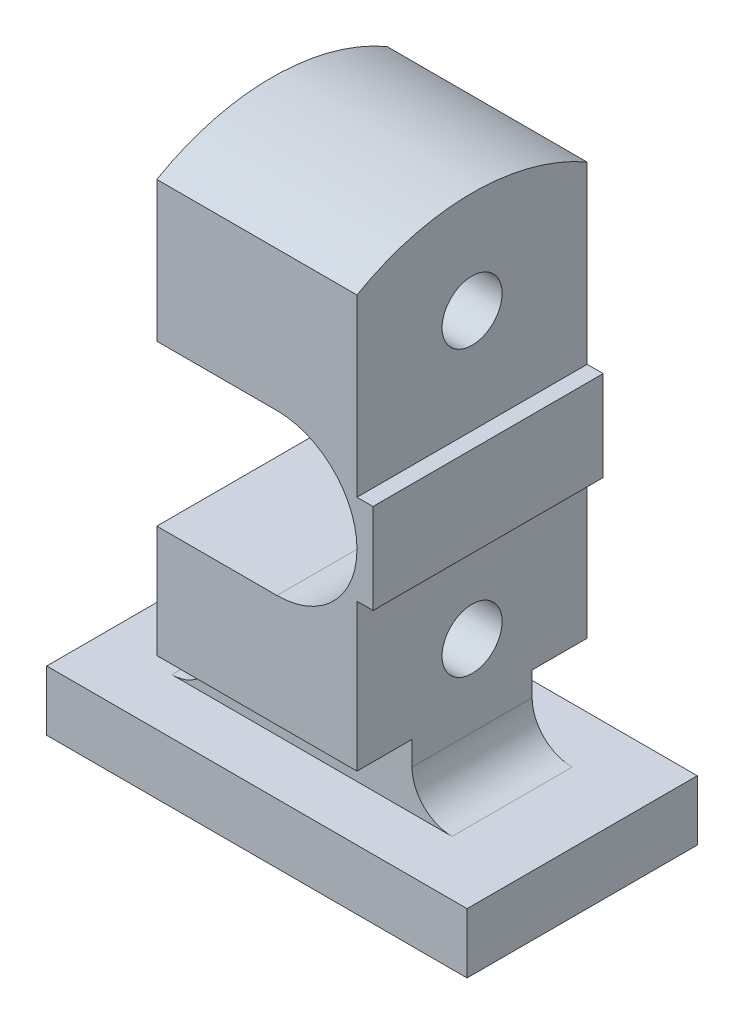
ISO-10303-21;
HEADER;
FILE_DESCRIPTION(('STEP AP214'),'2;1');
FILE_NAME('part.step','',(''),(''),'','','');
FILE_SCHEMA(('AUTOMOTIVE_DESIGN { 1 0 10303 214 1 1 1 1 }'));
ENDSEC;
DATA;
#1=APPLICATION_CONTEXT('core data for automotive mechanical design processes');
#2=APPLICATION_PROTOCOL_DEFINITION('international standard','automotive_design',2000,#1);
#3=PRODUCT_CONTEXT('',#1,'mechanical');
#4=PRODUCT('Part','Part','',(#3));
#5=PRODUCT_RELATED_PRODUCT_CATEGORY('part','',(#4));
#6=PRODUCT_DEFINITION_FORMATION('','',#4);
#7=PRODUCT_DEFINITION_CONTEXT('part definition',#1,'design');
#8=PRODUCT_DEFINITION('design','',#6,#7);
#9=PRODUCT_DEFINITION_SHAPE('','',#8);
#10=(LENGTH_UNIT() NAMED_UNIT(*) SI_UNIT(.MILLI.,.METRE.));
#11=(NAMED_UNIT(*) PLANE_ANGLE_UNIT() SI_UNIT($,.RADIAN.));
#12=(NAMED_UNIT(*) SI_UNIT($,.STERADIAN.) SOLID_ANGLE_UNIT());
#13=UNCERTAINTY_MEASURE_WITH_UNIT(LENGTH_MEASURE(1.E-05),#10,'distance_accuracy_value','');
#14=(GEOMETRIC_REPRESENTATION_CONTEXT(3) GLOBAL_UNCERTAINTY_ASSIGNED_CONTEXT((#13)) GLOBAL_UNIT_ASSIGNED_CONTEXT((#10,
#11,#12)) REPRESENTATION_CONTEXT('',''));
#15=CARTESIAN_POINT('',(0.,0.,0.));
#16=DIRECTION('',(0.,0.,1.));
#17=DIRECTION('',(1.,0.,0.));
#18=AXIS2_PLACEMENT_3D('',#15,#16,#17);
#19=CARTESIAN_POINT('',(0.,30.,0.));
#20=DIRECTION('',(0.,-1.,0.));
#21=DIRECTION('',(0.,0.,-1.));
#22=AXIS2_PLACEMENT_3D('',#19,#20,#21);
#23=PLANE('',#22);
#24=DIRECTION('',(0.,0.,-1.));
#25=VECTOR('',#24,1.);
#26=CARTESIAN_POINT('',(105.,30.,57.5));
#27=LINE('',#26,#25);
#28=CARTESIAN_POINT('',(105.,30.,57.5));
#29=VERTEX_POINT('',#28);
#30=CARTESIAN_POINT('',(105.,30.,-57.5));
#31=VERTEX_POINT('',#30);
#32=EDGE_CURVE('E323',#29,#31,#27,.T.);
#33=ORIENTED_EDGE('',*,*,#32,.T.);
#34=DIRECTION('',(-1.,0.,0.));
#35=VECTOR('',#34,1.);
#36=CARTESIAN_POINT('',(-105.,30.,-57.5));
#37=LINE('',#36,#35);
#38=CARTESIAN_POINT('',(-105.,30.,-57.5));
#39=VERTEX_POINT('',#38);
#40=EDGE_CURVE('E328',#31,#39,#37,.T.);
#41=ORIENTED_EDGE('',*,*,#40,.T.);
#42=DIRECTION('',(0.,0.,1.));
#43=VECTOR('',#42,1.);
#44=CARTESIAN_POINT('',(-105.,30.,57.5));
#45=LINE('',#44,#43);
#46=CARTESIAN_POINT('',(-105.,30.,57.5));
#47=VERTEX_POINT('',#46);
#48=EDGE_CURVE('E333',#39,#47,#45,.T.);
#49=ORIENTED_EDGE('',*,*,#48,.T.);
#50=DIRECTION('',(1.,0.,0.));
#51=VECTOR('',#50,1.);
#52=CARTESIAN_POINT('',(-105.,30.,57.5));
#53=LINE('',#52,#51);
#54=EDGE_CURVE('E332',#47,#29,#53,.T.);
#55=ORIENTED_EDGE('',*,*,#54,.T.);
#56=EDGE_LOOP('',(#33,#41,#49,#55));
#57=FACE_BOUND('',#56,.T.);
#58=DIRECTION('',(-1.,0.,0.));
#59=VECTOR('',#58,1.);
#60=CARTESIAN_POINT('',(-50.,30.,-30.));
#61=LINE('',#60,#59);
#62=CARTESIAN_POINT('',(70.,30.,-30.));
#63=VERTEX_POINT('',#62);
#64=CARTESIAN_POINT('',(-70.,30.,-30.));
#65=VERTEX_POINT('',#64);
#66=EDGE_CURVE('E303',#63,#65,#61,.T.);
#67=ORIENTED_EDGE('',*,*,#66,.F.);
#68=DIRECTION('',(0.,0.,-1.));
#69=VECTOR('',#68,1.);
#70=CARTESIAN_POINT('',(70.,30.,30.));
#71=LINE('',#70,#69);
#72=CARTESIAN_POINT('',(70.,30.,30.));
#73=VERTEX_POINT('',#72);
#74=EDGE_CURVE('E359',#63,#73,#71,.F.);
#75=ORIENTED_EDGE('',*,*,#74,.T.);
#76=DIRECTION('',(1.,0.,0.));
#77=VECTOR('',#76,1.);
#78=CARTESIAN_POINT('',(-50.,30.,30.));
#79=LINE('',#78,#77);
#80=CARTESIAN_POINT('',(-70.,30.,30.));
#81=VERTEX_POINT('',#80);
#82=EDGE_CURVE('E308',#81,#73,#79,.T.);
#83=ORIENTED_EDGE('',*,*,#82,.F.);
#84=DIRECTION('',(0.,0.,1.));
#85=VECTOR('',#84,1.);
#86=CARTESIAN_POINT('',(-70.,30.,-30.));
#87=LINE('',#86,#85);
#88=EDGE_CURVE('E357',#81,#65,#87,.F.);
#89=ORIENTED_EDGE('',*,*,#88,.T.);
#90=EDGE_LOOP('',(#67,#75,#83,#89));
#91=FACE_BOUND('',#90,.T.);
#92=ADVANCED_FACE('F39',(#57,#91),#23,.F.);
#93=CARTESIAN_POINT('',(105.,30.,57.5));
#94=DIRECTION('',(-1.,0.,0.));
#95=DIRECTION('',(0.,0.,1.));
#96=AXIS2_PLACEMENT_3D('',#93,#94,#95);
#97=PLANE('',#96);
#98=DIRECTION('',(0.,0.,-1.));
#99=VECTOR('',#98,1.);
#100=CARTESIAN_POINT('',(105.,0.,57.5));
#101=LINE('',#100,#99);
#102=CARTESIAN_POINT('',(105.,0.,57.5));
#103=VERTEX_POINT('',#102);
#104=CARTESIAN_POINT('',(105.,0.,-57.5));
#105=VERTEX_POINT('',#104);
#106=EDGE_CURVE('E321',#103,#105,#101,.T.);
#107=ORIENTED_EDGE('',*,*,#106,.T.);
#108=DIRECTION('',(0.,-1.,0.));
#109=VECTOR('',#108,1.);
#110=CARTESIAN_POINT('',(105.,30.,-57.5));
#111=LINE('',#110,#109);
#112=EDGE_CURVE('E353',#31,#105,#111,.T.);
#113=ORIENTED_EDGE('',*,*,#112,.F.);
#114=ORIENTED_EDGE('',*,*,#32,.F.);
#115=DIRECTION('',(0.,-1.,0.));
#116=VECTOR('',#115,1.);
#117=CARTESIAN_POINT('',(105.,30.,57.5));
#118=LINE('',#117,#116);
#119=EDGE_CURVE('E331',#29,#103,#118,.T.);
#120=ORIENTED_EDGE('',*,*,#119,.T.);
#121=EDGE_LOOP('',(#107,#113,#114,#120));
#122=FACE_BOUND('',#121,.T.);
#123=ADVANCED_FACE('F441',(#122),#97,.F.);
#124=CARTESIAN_POINT('',(-105.,30.,-57.5));
#125=DIRECTION('',(0.,0.,1.));
#126=DIRECTION('',(1.,0.,0.));
#127=AXIS2_PLACEMENT_3D('',#124,#125,#126);
#128=PLANE('',#127);
#129=DIRECTION('',(-1.,0.,0.));
#130=VECTOR('',#129,1.);
#131=CARTESIAN_POINT('',(-105.,0.,-57.5));
#132=LINE('',#131,#130);
#133=CARTESIAN_POINT('',(-105.,0.,-57.5));
#134=VERTEX_POINT('',#133);
#135=EDGE_CURVE('E336',#105,#134,#132,.T.);
#136=ORIENTED_EDGE('',*,*,#135,.T.);
#137=DIRECTION('',(0.,-1.,0.));
#138=VECTOR('',#137,1.);
#139=CARTESIAN_POINT('',(-105.,30.,-57.5));
#140=LINE('',#139,#138);
#141=EDGE_CURVE('E348',#39,#134,#140,.T.);
#142=ORIENTED_EDGE('',*,*,#141,.F.);
#143=ORIENTED_EDGE('',*,*,#40,.F.);
#144=ORIENTED_EDGE('',*,*,#112,.T.);
#145=EDGE_LOOP('',(#136,#142,#143,#144));
#146=FACE_BOUND('',#145,.T.);
#147=ADVANCED_FACE('F446',(#146),#128,.F.);
#148=CARTESIAN_POINT('',(-105.,30.,57.5));
#149=DIRECTION('',(1.,0.,0.));
#150=DIRECTION('',(0.,0.,-1.));
#151=AXIS2_PLACEMENT_3D('',#148,#149,#150);
#152=PLANE('',#151);
#153=DIRECTION('',(0.,0.,1.));
#154=VECTOR('',#153,1.);
#155=CARTESIAN_POINT('',(-105.,0.,57.5));
#156=LINE('',#155,#154);
#157=CARTESIAN_POINT('',(-105.,0.,57.5));
#158=VERTEX_POINT('',#157);
#159=EDGE_CURVE('E338',#134,#158,#156,.T.);
#160=ORIENTED_EDGE('',*,*,#159,.T.);
#161=DIRECTION('',(0.,-1.,0.));
#162=VECTOR('',#161,1.);
#163=CARTESIAN_POINT('',(-105.,30.,57.5));
#164=LINE('',#163,#162);
#165=EDGE_CURVE('E343',#47,#158,#164,.T.);
#166=ORIENTED_EDGE('',*,*,#165,.F.);
#167=ORIENTED_EDGE('',*,*,#48,.F.);
#168=ORIENTED_EDGE('',*,*,#141,.T.);
#169=EDGE_LOOP('',(#160,#166,#167,#168));
#170=FACE_BOUND('',#169,.T.);
#171=ADVANCED_FACE('F463',(#170),#152,.F.);
#172=CARTESIAN_POINT('',(-105.,30.,57.5));
#173=DIRECTION('',(0.,0.,-1.));
#174=DIRECTION('',(-1.,0.,0.));
#175=AXIS2_PLACEMENT_3D('',#172,#173,#174);
#176=PLANE('',#175);
#177=DIRECTION('',(1.,0.,0.));
#178=VECTOR('',#177,1.);
#179=CARTESIAN_POINT('',(-105.,0.,57.5));
#180=LINE('',#179,#178);
#181=EDGE_CURVE('E329',#158,#103,#180,.T.);
#182=ORIENTED_EDGE('',*,*,#181,.T.);
#183=ORIENTED_EDGE('',*,*,#119,.F.);
#184=ORIENTED_EDGE('',*,*,#54,.F.);
#185=ORIENTED_EDGE('',*,*,#165,.T.);
#186=EDGE_LOOP('',(#182,#183,#184,#185));
#187=FACE_BOUND('',#186,.T.);
#188=ADVANCED_FACE('F460',(#187),#176,.F.);
#189=CARTESIAN_POINT('',(0.,0.,0.));
#190=DIRECTION('',(0.,-1.,0.));
#191=DIRECTION('',(0.,0.,-1.));
#192=AXIS2_PLACEMENT_3D('',#189,#190,#191);
#193=PLANE('',#192);
#194=ORIENTED_EDGE('',*,*,#106,.F.);
#195=ORIENTED_EDGE('',*,*,#181,.F.);
#196=ORIENTED_EDGE('',*,*,#159,.F.);
#197=ORIENTED_EDGE('',*,*,#135,.F.);
#198=EDGE_LOOP('',(#194,#195,#196,#197));
#199=FACE_BOUND('',#198,.T.);
#200=ADVANCED_FACE('F453',(#199),#193,.T.);
#201=CARTESIAN_POINT('',(50.,62.,30.));
#202=DIRECTION('',(-1.,0.,0.));
#203=DIRECTION('',(0.,0.,1.));
#204=AXIS2_PLACEMENT_3D('',#201,#202,#203);
#205=PLANE('',#204);
#206=CARTESIAN_POINT('',(50.,90.5,0.));
#207=DIRECTION('',(-1.,0.,0.));
#208=DIRECTION('',(0.,0.,1.));
#209=AXIS2_PLACEMENT_3D('',#206,#207,#208);
#210=CIRCLE('',#209,15.);
#211=CARTESIAN_POINT('',(50.,90.5,15.));
#212=VERTEX_POINT('',#211);
#213=EDGE_CURVE('E225',#212,#212,#210,.T.);
#214=ORIENTED_EDGE('',*,*,#213,.T.);
#215=EDGE_LOOP('',(#214));
#216=FACE_BOUND('',#215,.T.);
#217=DIRECTION('',(0.,-1.,0.));
#218=VECTOR('',#217,1.);
#219=CARTESIAN_POINT('',(50.,62.,30.));
#220=LINE('',#219,#218);
#221=CARTESIAN_POINT('',(50.,62.,30.));
#222=VERTEX_POINT('',#221);
#223=CARTESIAN_POINT('',(50.,50.,30.));
#224=VERTEX_POINT('',#223);
#225=EDGE_CURVE('E311',#222,#224,#220,.T.);
#226=ORIENTED_EDGE('',*,*,#225,.T.);
#227=DIRECTION('',(0.,0.,-1.));
#228=VECTOR('',#227,1.);
#229=CARTESIAN_POINT('',(50.,50.,-30.));
#230=LINE('',#229,#228);
#231=CARTESIAN_POINT('',(50.,50.,-30.));
#232=VERTEX_POINT('',#231);
#233=EDGE_CURVE('E355',#224,#232,#230,.T.);
#234=ORIENTED_EDGE('',*,*,#233,.T.);
#235=DIRECTION('',(0.,-1.,0.));
#236=VECTOR('',#235,1.);
#237=CARTESIAN_POINT('',(50.,62.,-30.));
#238=LINE('',#237,#236);
#239=CARTESIAN_POINT('',(50.,62.,-30.));
#240=VERTEX_POINT('',#239);
#241=EDGE_CURVE('E322',#240,#232,#238,.T.);
#242=ORIENTED_EDGE('',*,*,#241,.F.);
#243=DIRECTION('',(0.,0.,-1.));
#244=VECTOR('',#243,1.);
#245=CARTESIAN_POINT('',(50.,62.,57.5));
#246=LINE('',#245,#244);
#247=CARTESIAN_POINT('',(50.,62.,-57.5));
#248=VERTEX_POINT('',#247);
#249=EDGE_CURVE('E299',#240,#248,#246,.T.);
#250=ORIENTED_EDGE('',*,*,#249,.T.);
#251=DIRECTION('',(0.,1.,0.));
#252=VECTOR('',#251,1.);
#253=CARTESIAN_POINT('',(50.,118.,-57.5));
#254=LINE('',#253,#252);
#255=CARTESIAN_POINT('',(50.,135.5,-57.5));
#256=VERTEX_POINT('',#255);
#257=EDGE_CURVE('E257',#248,#256,#254,.T.);
#258=ORIENTED_EDGE('',*,*,#257,.T.);
#259=DIRECTION('',(0.,0.,-1.));
#260=VECTOR('',#259,1.);
#261=CARTESIAN_POINT('',(50.,135.5,57.5));
#262=LINE('',#261,#260);
#263=CARTESIAN_POINT('',(50.,135.5,57.5));
#264=VERTEX_POINT('',#263);
#265=EDGE_CURVE('E298',#264,#256,#262,.T.);
#266=ORIENTED_EDGE('',*,*,#265,.F.);
#267=DIRECTION('',(0.,1.,0.));
#268=VECTOR('',#267,1.);
#269=CARTESIAN_POINT('',(50.,62.,57.5));
#270=LINE('',#269,#268);
#271=CARTESIAN_POINT('',(50.,62.,57.5));
#272=VERTEX_POINT('',#271);
#273=EDGE_CURVE('E233',#272,#264,#270,.T.);
#274=ORIENTED_EDGE('',*,*,#273,.F.);
#275=EDGE_CURVE('E297',#272,#222,#246,.T.);
#276=ORIENTED_EDGE('',*,*,#275,.T.);
#277=EDGE_LOOP('',(#226,#234,#242,#250,#258,#266,#274,#276));
#278=FACE_BOUND('',#277,.T.);
#279=ADVANCED_FACE('F378',(#216,#278),#205,.F.);
#280=CARTESIAN_POINT('',(-50.,62.,-30.));
#281=DIRECTION('',(0.,0.,1.));
#282=DIRECTION('',(1.,0.,0.));
#283=AXIS2_PLACEMENT_3D('',#280,#281,#282);
#284=PLANE('',#283);
#285=ORIENTED_EDGE('',*,*,#66,.T.);
#286=CARTESIAN_POINT('',(-70.,50.,-30.));
#287=DIRECTION('',(0.,0.,1.));
#288=DIRECTION('',(1.,0.,0.));
#289=AXIS2_PLACEMENT_3D('',#286,#287,#288);
#290=CIRCLE('',#289,20.);
#291=CARTESIAN_POINT('',(-50.,50.,-30.));
#292=VERTEX_POINT('',#291);
#293=EDGE_CURVE('E11',#65,#292,#290,.T.);
#294=ORIENTED_EDGE('',*,*,#293,.T.);
#295=DIRECTION('',(0.,-1.,0.));
#296=VECTOR('',#295,1.);
#297=CARTESIAN_POINT('',(-50.,62.,-30.));
#298=LINE('',#297,#296);
#299=CARTESIAN_POINT('',(-50.,62.,-30.));
#300=VERTEX_POINT('',#299);
#301=EDGE_CURVE('E316',#300,#292,#298,.T.);
#302=ORIENTED_EDGE('',*,*,#301,.F.);
#303=DIRECTION('',(-1.,0.,0.));
#304=VECTOR('',#303,1.);
#305=CARTESIAN_POINT('',(-50.,62.,-30.));
#306=LINE('',#305,#304);
#307=EDGE_CURVE('E302',#240,#300,#306,.T.);
#308=ORIENTED_EDGE('',*,*,#307,.F.);
#309=ORIENTED_EDGE('',*,*,#241,.T.);
#310=CARTESIAN_POINT('',(70.,50.,-30.));
#311=DIRECTION('',(0.,0.,1.));
#312=DIRECTION('',(1.,0.,0.));
#313=AXIS2_PLACEMENT_3D('',#310,#311,#312);
#314=CIRCLE('',#313,20.);
#315=EDGE_CURVE('E362',#232,#63,#314,.T.);
#316=ORIENTED_EDGE('',*,*,#315,.T.);
#317=EDGE_LOOP('',(#285,#294,#302,#308,#309,#316));
#318=FACE_BOUND('',#317,.T.);
#319=ADVANCED_FACE('F392',(#318),#284,.F.);
#320=CARTESIAN_POINT('',(-50.,62.,30.));
#321=DIRECTION('',(1.,0.,0.));
#322=DIRECTION('',(0.,0.,-1.));
#323=AXIS2_PLACEMENT_3D('',#320,#321,#322);
#324=PLANE('',#323);
#325=CARTESIAN_POINT('',(-50.,90.5,0.));
#326=DIRECTION('',(-1.,0.,0.));
#327=DIRECTION('',(0.,0.,1.));
#328=AXIS2_PLACEMENT_3D('',#325,#326,#327);
#329=CIRCLE('',#328,15.);
#330=CARTESIAN_POINT('',(-50.,90.5,15.));
#331=VERTEX_POINT('',#330);
#332=EDGE_CURVE('E217',#331,#331,#329,.T.);
#333=ORIENTED_EDGE('',*,*,#332,.F.);
#334=EDGE_LOOP('',(#333));
#335=FACE_BOUND('',#334,.T.);
#336=ORIENTED_EDGE('',*,*,#301,.T.);
#337=DIRECTION('',(0.,0.,1.));
#338=VECTOR('',#337,1.);
#339=CARTESIAN_POINT('',(-50.,50.,30.));
#340=LINE('',#339,#338);
#341=CARTESIAN_POINT('',(-50.,50.,30.));
#342=VERTEX_POINT('',#341);
#343=EDGE_CURVE('E361',#292,#342,#340,.T.);
#344=ORIENTED_EDGE('',*,*,#343,.T.);
#345=DIRECTION('',(0.,-1.,0.));
#346=VECTOR('',#345,1.);
#347=CARTESIAN_POINT('',(-50.,62.,30.));
#348=LINE('',#347,#346);
#349=CARTESIAN_POINT('',(-50.,62.,30.));
#350=VERTEX_POINT('',#349);
#351=EDGE_CURVE('E317',#350,#342,#348,.T.);
#352=ORIENTED_EDGE('',*,*,#351,.F.);
#353=DIRECTION('',(0.,0.,-1.));
#354=VECTOR('',#353,1.);
#355=CARTESIAN_POINT('',(-50.,62.,57.5));
#356=LINE('',#355,#354);
#357=CARTESIAN_POINT('',(-50.,62.,57.5));
#358=VERTEX_POINT('',#357);
#359=EDGE_CURVE('E271',#358,#350,#356,.T.);
#360=ORIENTED_EDGE('',*,*,#359,.F.);
#361=DIRECTION('',(0.,-1.,0.));
#362=VECTOR('',#361,1.);
#363=CARTESIAN_POINT('',(-50.,118.,57.5));
#364=LINE('',#363,#362);
#365=CARTESIAN_POINT('',(-50.,118.,57.5));
#366=VERTEX_POINT('',#365);
#367=EDGE_CURVE('E252',#366,#358,#364,.T.);
#368=ORIENTED_EDGE('',*,*,#367,.F.);
#369=DIRECTION('',(0.,0.,-1.));
#370=VECTOR('',#369,1.);
#371=CARTESIAN_POINT('',(-50.,118.,57.5));
#372=LINE('',#371,#370);
#373=CARTESIAN_POINT('',(-50.,118.,-57.5));
#374=VERTEX_POINT('',#373);
#375=EDGE_CURVE('E277',#366,#374,#372,.T.);
#376=ORIENTED_EDGE('',*,*,#375,.T.);
#377=DIRECTION('',(0.,-1.,0.));
#378=VECTOR('',#377,1.);
#379=CARTESIAN_POINT('',(-50.,118.,-57.5));
#380=LINE('',#379,#378);
#381=CARTESIAN_POINT('',(-50.,62.,-57.5));
#382=VERTEX_POINT('',#381);
#383=EDGE_CURVE('E235',#374,#382,#380,.T.);
#384=ORIENTED_EDGE('',*,*,#383,.T.);
#385=EDGE_CURVE('E254',#300,#382,#356,.T.);
#386=ORIENTED_EDGE('',*,*,#385,.F.);
#387=EDGE_LOOP('',(#336,#344,#352,#360,#368,#376,#384,#386));
#388=FACE_BOUND('',#387,.T.);
#389=ADVANCED_FACE('F386',(#335,#388),#324,.F.);
#390=CARTESIAN_POINT('',(-50.,62.,30.));
#391=DIRECTION('',(0.,0.,-1.));
#392=DIRECTION('',(-1.,0.,0.));
#393=AXIS2_PLACEMENT_3D('',#390,#391,#392);
#394=PLANE('',#393);
#395=ORIENTED_EDGE('',*,*,#82,.T.);
#396=CARTESIAN_POINT('',(70.,50.,30.));
#397=DIRECTION('',(0.,0.,-1.));
#398=DIRECTION('',(-1.,0.,0.));
#399=AXIS2_PLACEMENT_3D('',#396,#397,#398);
#400=CIRCLE('',#399,20.);
#401=EDGE_CURVE('E368',#73,#224,#400,.T.);
#402=ORIENTED_EDGE('',*,*,#401,.T.);
#403=ORIENTED_EDGE('',*,*,#225,.F.);
#404=DIRECTION('',(1.,0.,0.));
#405=VECTOR('',#404,1.);
#406=CARTESIAN_POINT('',(-50.,62.,30.));
#407=LINE('',#406,#405);
#408=EDGE_CURVE('E310',#350,#222,#407,.T.);
#409=ORIENTED_EDGE('',*,*,#408,.F.);
#410=ORIENTED_EDGE('',*,*,#351,.T.);
#411=CARTESIAN_POINT('',(-70.,50.,30.));
#412=DIRECTION('',(0.,0.,-1.));
#413=DIRECTION('',(-1.,0.,0.));
#414=AXIS2_PLACEMENT_3D('',#411,#412,#413);
#415=CIRCLE('',#414,20.);
#416=EDGE_CURVE('E50',#342,#81,#415,.T.);
#417=ORIENTED_EDGE('',*,*,#416,.T.);
#418=EDGE_LOOP('',(#395,#402,#403,#409,#410,#417));
#419=FACE_BOUND('',#418,.T.);
#420=ADVANCED_FACE('F369',(#419),#394,.F.);
#421=CARTESIAN_POINT('',(70.,50.,30.));
#422=DIRECTION('',(0.,0.,1.));
#423=DIRECTION('',(1.,0.,0.));
#424=AXIS2_PLACEMENT_3D('',#421,#422,#423);
#425=CYLINDRICAL_SURFACE('',#424,20.);
#426=ORIENTED_EDGE('',*,*,#401,.F.);
#427=ORIENTED_EDGE('',*,*,#74,.F.);
#428=ORIENTED_EDGE('',*,*,#315,.F.);
#429=ORIENTED_EDGE('',*,*,#233,.F.);
#430=EDGE_LOOP('',(#426,#427,#428,#429));
#431=FACE_BOUND('',#430,.T.);
#432=ADVANCED_FACE('F380',(#431),#425,.F.);
#433=CARTESIAN_POINT('',(-70.,50.,30.));
#434=DIRECTION('',(0.,0.,-1.));
#435=DIRECTION('',(-1.,0.,0.));
#436=AXIS2_PLACEMENT_3D('',#433,#434,#435);
#437=CYLINDRICAL_SURFACE('',#436,20.);
#438=ORIENTED_EDGE('',*,*,#293,.F.);
#439=ORIENTED_EDGE('',*,*,#88,.F.);
#440=ORIENTED_EDGE('',*,*,#416,.F.);
#441=ORIENTED_EDGE('',*,*,#343,.F.);
#442=EDGE_LOOP('',(#438,#439,#440,#441));
#443=FACE_BOUND('',#442,.T.);
#444=ADVANCED_FACE('F41',(#443),#437,.F.);
#445=CARTESIAN_POINT('',(-50.,62.,57.5));
#446=DIRECTION('',(0.,1.,0.));
#447=DIRECTION('',(0.,0.,1.));
#448=AXIS2_PLACEMENT_3D('',#445,#446,#447);
#449=PLANE('',#448);
#450=ORIENTED_EDGE('',*,*,#249,.F.);
#451=ORIENTED_EDGE('',*,*,#307,.T.);
#452=ORIENTED_EDGE('',*,*,#385,.T.);
#453=DIRECTION('',(1.,0.,0.));
#454=VECTOR('',#453,1.);
#455=CARTESIAN_POINT('',(-50.,62.,-57.5));
#456=LINE('',#455,#454);
#457=EDGE_CURVE('E227',#382,#248,#456,.T.);
#458=ORIENTED_EDGE('',*,*,#457,.T.);
#459=EDGE_LOOP('',(#450,#451,#452,#458));
#460=FACE_BOUND('',#459,.T.);
#461=ADVANCED_FACE('F394',(#460),#449,.F.);
#462=ORIENTED_EDGE('',*,*,#359,.T.);
#463=ORIENTED_EDGE('',*,*,#408,.T.);
#464=ORIENTED_EDGE('',*,*,#275,.F.);
#465=DIRECTION('',(1.,0.,0.));
#466=VECTOR('',#465,1.);
#467=CARTESIAN_POINT('',(-50.,62.,57.5));
#468=LINE('',#467,#466);
#469=EDGE_CURVE('E226',#358,#272,#468,.T.);
#470=ORIENTED_EDGE('',*,*,#469,.F.);
#471=EDGE_LOOP('',(#462,#463,#464,#470));
#472=FACE_BOUND('',#471,.T.);
#473=ADVANCED_FACE('F383',(#472),#449,.F.);
#474=CARTESIAN_POINT('',(50.,135.5,57.5));
#475=DIRECTION('',(0.,1.,0.));
#476=DIRECTION('',(0.,0.,1.));
#477=AXIS2_PLACEMENT_3D('',#474,#475,#476);
#478=PLANE('',#477);
#479=DIRECTION('',(1.,0.,0.));
#480=VECTOR('',#479,1.);
#481=CARTESIAN_POINT('',(50.,135.5,-57.5));
#482=LINE('',#481,#480);
#483=CARTESIAN_POINT('',(58.,135.5,-57.5));
#484=VERTEX_POINT('',#483);
#485=EDGE_CURVE('E259',#256,#484,#482,.T.);
#486=ORIENTED_EDGE('',*,*,#485,.T.);
#487=DIRECTION('',(0.,0.,-1.));
#488=VECTOR('',#487,1.);
#489=CARTESIAN_POINT('',(58.,135.5,57.5));
#490=LINE('',#489,#488);
#491=CARTESIAN_POINT('',(58.,135.5,57.5));
#492=VERTEX_POINT('',#491);
#493=EDGE_CURVE('E291',#492,#484,#490,.T.);
#494=ORIENTED_EDGE('',*,*,#493,.F.);
#495=DIRECTION('',(1.,0.,0.));
#496=VECTOR('',#495,1.);
#497=CARTESIAN_POINT('',(50.,135.5,57.5));
#498=LINE('',#497,#496);
#499=EDGE_CURVE('E234',#264,#492,#498,.T.);
#500=ORIENTED_EDGE('',*,*,#499,.F.);
#501=ORIENTED_EDGE('',*,*,#265,.T.);
#502=EDGE_LOOP('',(#486,#494,#500,#501));
#503=FACE_BOUND('',#502,.T.);
#504=ADVANCED_FACE('F405',(#503),#478,.F.);
#505=CARTESIAN_POINT('',(58.,135.5,57.5));
#506=DIRECTION('',(-1.,0.,0.));
#507=DIRECTION('',(0.,0.,1.));
#508=AXIS2_PLACEMENT_3D('',#505,#506,#507);
#509=PLANE('',#508);
#510=DIRECTION('',(0.,1.,0.));
#511=VECTOR('',#510,1.);
#512=CARTESIAN_POINT('',(58.,135.5,-57.5));
#513=LINE('',#512,#511);
#514=CARTESIAN_POINT('',(58.,180.5,-57.5));
#515=VERTEX_POINT('',#514);
#516=EDGE_CURVE('E258',#484,#515,#513,.T.);
#517=ORIENTED_EDGE('',*,*,#516,.T.);
#518=DIRECTION('',(0.,0.,-1.));
#519=VECTOR('',#518,1.);
#520=CARTESIAN_POINT('',(58.,180.5,57.5));
#521=LINE('',#520,#519);
#522=CARTESIAN_POINT('',(58.,180.5,57.5));
#523=VERTEX_POINT('',#522);
#524=EDGE_CURVE('E286',#523,#515,#521,.T.);
#525=ORIENTED_EDGE('',*,*,#524,.F.);
#526=DIRECTION('',(0.,1.,0.));
#527=VECTOR('',#526,1.);
#528=CARTESIAN_POINT('',(58.,135.5,57.5));
#529=LINE('',#528,#527);
#530=EDGE_CURVE('E236',#492,#523,#529,.T.);
#531=ORIENTED_EDGE('',*,*,#530,.F.);
#532=ORIENTED_EDGE('',*,*,#493,.T.);
#533=EDGE_LOOP('',(#517,#525,#531,#532));
#534=FACE_BOUND('',#533,.T.);
#535=ADVANCED_FACE('F407',(#534),#509,.F.);
#536=CARTESIAN_POINT('',(58.,180.5,57.5));
#537=DIRECTION('',(0.,-1.,0.));
#538=DIRECTION('',(0.,0.,-1.));
#539=AXIS2_PLACEMENT_3D('',#536,#537,#538);
#540=PLANE('',#539);
#541=DIRECTION('',(-1.,0.,0.));
#542=VECTOR('',#541,1.);
#543=CARTESIAN_POINT('',(58.,180.5,-57.5));
#544=LINE('',#543,#542);
#545=CARTESIAN_POINT('',(50.,180.5,-57.5));
#546=VERTEX_POINT('',#545);
#547=EDGE_CURVE('E265',#515,#546,#544,.T.);
#548=ORIENTED_EDGE('',*,*,#547,.T.);
#549=DIRECTION('',(0.,0.,-1.));
#550=VECTOR('',#549,1.);
#551=CARTESIAN_POINT('',(50.,180.5,57.5));
#552=LINE('',#551,#550);
#553=CARTESIAN_POINT('',(50.,180.5,57.5));
#554=VERTEX_POINT('',#553);
#555=EDGE_CURVE('E289',#554,#546,#552,.T.);
#556=ORIENTED_EDGE('',*,*,#555,.F.);
#557=DIRECTION('',(-1.,0.,0.));
#558=VECTOR('',#557,1.);
#559=CARTESIAN_POINT('',(58.,180.5,57.5));
#560=LINE('',#559,#558);
#561=EDGE_CURVE('E238',#523,#554,#560,.T.);
#562=ORIENTED_EDGE('',*,*,#561,.F.);
#563=ORIENTED_EDGE('',*,*,#524,.T.);
#564=EDGE_LOOP('',(#548,#556,#562,#563));
#565=FACE_BOUND('',#564,.T.);
#566=ADVANCED_FACE('F429',(#565),#540,.F.);
#567=CARTESIAN_POINT('',(50.,198.,57.5));
#568=DIRECTION('',(-1.,0.,0.));
#569=DIRECTION('',(0.,0.,1.));
#570=AXIS2_PLACEMENT_3D('',#567,#568,#569);
#571=PLANE('',#570);
#572=CARTESIAN_POINT('',(50.,232.5,0.));
#573=DIRECTION('',(-1.,0.,0.));
#574=DIRECTION('',(0.,0.,1.));
#575=AXIS2_PLACEMENT_3D('',#572,#573,#574);
#576=CIRCLE('',#575,15.);
#577=CARTESIAN_POINT('',(50.,232.5,15.));
#578=VERTEX_POINT('',#577);
#579=EDGE_CURVE('E219',#578,#578,#576,.T.);
#580=ORIENTED_EDGE('',*,*,#579,.T.);
#581=EDGE_LOOP('',(#580));
#582=FACE_BOUND('',#581,.T.);
#583=DIRECTION('',(0.,1.,0.));
#584=VECTOR('',#583,1.);
#585=CARTESIAN_POINT('',(50.,198.,-57.5));
#586=LINE('',#585,#584);
#587=CARTESIAN_POINT('',(50.,268.,-57.5));
#588=VERTEX_POINT('',#587);
#589=EDGE_CURVE('E210',#546,#588,#586,.T.);
#590=ORIENTED_EDGE('',*,*,#589,.T.);
#591=CARTESIAN_POINT('',(50.,168.40707856479,0.));
#592=DIRECTION('',(-1.,0.,0.));
#593=DIRECTION('',(0.,0.,-1.));
#594=AXIS2_PLACEMENT_3D('',#591,#592,#593);
#595=CIRCLE('',#594,115.);
#596=CARTESIAN_POINT('',(50.,268.,57.5));
#597=VERTEX_POINT('',#596);
#598=EDGE_CURVE('E207',#597,#588,#595,.T.);
#599=ORIENTED_EDGE('',*,*,#598,.F.);
#600=DIRECTION('',(0.,1.,0.));
#601=VECTOR('',#600,1.);
#602=CARTESIAN_POINT('',(50.,180.5,57.5));
#603=LINE('',#602,#601);
#604=EDGE_CURVE('E239',#554,#597,#603,.T.);
#605=ORIENTED_EDGE('',*,*,#604,.F.);
#606=ORIENTED_EDGE('',*,*,#555,.T.);
#607=EDGE_LOOP('',(#590,#599,#605,#606));
#608=FACE_BOUND('',#607,.T.);
#609=ADVANCED_FACE('F430',(#582,#608),#571,.F.);
#610=CARTESIAN_POINT('',(-50.,268.,57.5));
#611=DIRECTION('',(1.,0.,0.));
#612=DIRECTION('',(0.,0.,-1.));
#613=AXIS2_PLACEMENT_3D('',#610,#611,#612);
#614=PLANE('',#613);
#615=CARTESIAN_POINT('',(-50.,232.5,0.));
#616=DIRECTION('',(-1.,0.,0.));
#617=DIRECTION('',(0.,0.,1.));
#618=AXIS2_PLACEMENT_3D('',#615,#616,#617);
#619=CIRCLE('',#618,15.);
#620=CARTESIAN_POINT('',(-50.,232.5,15.));
#621=VERTEX_POINT('',#620);
#622=EDGE_CURVE('E214',#621,#621,#619,.T.);
#623=ORIENTED_EDGE('',*,*,#622,.F.);
#624=EDGE_LOOP('',(#623));
#625=FACE_BOUND('',#624,.T.);
#626=DIRECTION('',(0.,-1.,0.));
#627=VECTOR('',#626,1.);
#628=CARTESIAN_POINT('',(-50.,268.,-57.5));
#629=LINE('',#628,#627);
#630=CARTESIAN_POINT('',(-50.,268.,-57.5));
#631=VERTEX_POINT('',#630);
#632=CARTESIAN_POINT('',(-50.,198.,-57.5));
#633=VERTEX_POINT('',#632);
#634=EDGE_CURVE('E190',#631,#633,#629,.T.);
#635=ORIENTED_EDGE('',*,*,#634,.T.);
#636=DIRECTION('',(0.,0.,-1.));
#637=VECTOR('',#636,1.);
#638=CARTESIAN_POINT('',(-50.,198.,57.5));
#639=LINE('',#638,#637);
#640=CARTESIAN_POINT('',(-50.,198.,57.5));
#641=VERTEX_POINT('',#640);
#642=EDGE_CURVE('E281',#641,#633,#639,.T.);
#643=ORIENTED_EDGE('',*,*,#642,.F.);
#644=DIRECTION('',(0.,-1.,0.));
#645=VECTOR('',#644,1.);
#646=CARTESIAN_POINT('',(-50.,268.,57.5));
#647=LINE('',#646,#645);
#648=CARTESIAN_POINT('',(-50.,268.,57.5));
#649=VERTEX_POINT('',#648);
#650=EDGE_CURVE('E212',#649,#641,#647,.T.);
#651=ORIENTED_EDGE('',*,*,#650,.F.);
#652=CARTESIAN_POINT('',(-50.,168.40707856479,0.));
#653=DIRECTION('',(-1.,0.,0.));
#654=DIRECTION('',(0.,0.,-1.));
#655=AXIS2_PLACEMENT_3D('',#652,#653,#654);
#656=CIRCLE('',#655,115.);
#657=EDGE_CURVE('E205',#649,#631,#656,.T.);
#658=ORIENTED_EDGE('',*,*,#657,.T.);
#659=EDGE_LOOP('',(#635,#643,#651,#658));
#660=FACE_BOUND('',#659,.T.);
#661=ADVANCED_FACE('F208',(#625,#660),#614,.F.);
#662=CARTESIAN_POINT('',(-50.,198.,57.5));
#663=DIRECTION('',(0.,1.,0.));
#664=DIRECTION('',(0.,0.,1.));
#665=AXIS2_PLACEMENT_3D('',#662,#663,#664);
#666=PLANE('',#665);
#667=DIRECTION('',(1.,0.,0.));
#668=VECTOR('',#667,1.);
#669=CARTESIAN_POINT('',(-50.,198.,-57.5));
#670=LINE('',#669,#668);
#671=CARTESIAN_POINT('',(10.,198.,-57.5));
#672=VERTEX_POINT('',#671);
#673=EDGE_CURVE('E191',#633,#672,#670,.T.);
#674=ORIENTED_EDGE('',*,*,#673,.T.);
#675=DIRECTION('',(0.,0.,-1.));
#676=VECTOR('',#675,1.);
#677=CARTESIAN_POINT('',(10.,198.,57.5));
#678=LINE('',#677,#676);
#679=CARTESIAN_POINT('',(10.,198.,57.5));
#680=VERTEX_POINT('',#679);
#681=EDGE_CURVE('E285',#680,#672,#678,.T.);
#682=ORIENTED_EDGE('',*,*,#681,.F.);
#683=DIRECTION('',(1.,0.,0.));
#684=VECTOR('',#683,1.);
#685=CARTESIAN_POINT('',(-50.,198.,57.5));
#686=LINE('',#685,#684);
#687=EDGE_CURVE('E244',#641,#680,#686,.T.);
#688=ORIENTED_EDGE('',*,*,#687,.F.);
#689=ORIENTED_EDGE('',*,*,#642,.T.);
#690=EDGE_LOOP('',(#674,#682,#688,#689));
#691=FACE_BOUND('',#690,.T.);
#692=ADVANCED_FACE('F425',(#691),#666,.F.);
#693=CARTESIAN_POINT('',(10.,158.,57.5));
#694=DIRECTION('',(0.,0.,-1.));
#695=DIRECTION('',(-1.,0.,0.));
#696=AXIS2_PLACEMENT_3D('',#693,#694,#695);
#697=CYLINDRICAL_SURFACE('',#696,40.);
#698=CARTESIAN_POINT('',(10.,158.,-57.5));
#699=DIRECTION('',(0.,0.,-1.));
#700=DIRECTION('',(1.,0.,0.));
#701=AXIS2_PLACEMENT_3D('',#698,#699,#700);
#702=CIRCLE('',#701,40.);
#703=CARTESIAN_POINT('',(10.,118.,-57.5));
#704=VERTEX_POINT('',#703);
#705=EDGE_CURVE('E269',#672,#704,#702,.T.);
#706=ORIENTED_EDGE('',*,*,#705,.T.);
#707=DIRECTION('',(0.,0.,-1.));
#708=VECTOR('',#707,1.);
#709=CARTESIAN_POINT('',(10.,118.,57.5));
#710=LINE('',#709,#708);
#711=CARTESIAN_POINT('',(10.,118.,57.5));
#712=VERTEX_POINT('',#711);
#713=EDGE_CURVE('E276',#712,#704,#710,.T.);
#714=ORIENTED_EDGE('',*,*,#713,.F.);
#715=CARTESIAN_POINT('',(10.,158.,57.5));
#716=DIRECTION('',(0.,0.,-1.));
#717=DIRECTION('',(1.,0.,0.));
#718=AXIS2_PLACEMENT_3D('',#715,#716,#717);
#719=CIRCLE('',#718,40.);
#720=EDGE_CURVE('E250',#680,#712,#719,.T.);
#721=ORIENTED_EDGE('',*,*,#720,.F.);
#722=ORIENTED_EDGE('',*,*,#681,.T.);
#723=EDGE_LOOP('',(#706,#714,#721,#722));
#724=FACE_BOUND('',#723,.T.);
#725=ADVANCED_FACE('F416',(#724),#697,.F.);
#726=CARTESIAN_POINT('',(10.,118.,57.5));
#727=DIRECTION('',(0.,-1.,0.));
#728=DIRECTION('',(0.,0.,-1.));
#729=AXIS2_PLACEMENT_3D('',#726,#727,#728);
#730=PLANE('',#729);
#731=DIRECTION('',(-1.,0.,0.));
#732=VECTOR('',#731,1.);
#733=CARTESIAN_POINT('',(10.,118.,-57.5));
#734=LINE('',#733,#732);
#735=EDGE_CURVE('E270',#704,#374,#734,.T.);
#736=ORIENTED_EDGE('',*,*,#735,.T.);
#737=ORIENTED_EDGE('',*,*,#375,.F.);
#738=DIRECTION('',(-1.,0.,0.));
#739=VECTOR('',#738,1.);
#740=CARTESIAN_POINT('',(10.,118.,57.5));
#741=LINE('',#740,#739);
#742=EDGE_CURVE('E248',#712,#366,#741,.T.);
#743=ORIENTED_EDGE('',*,*,#742,.F.);
#744=ORIENTED_EDGE('',*,*,#713,.T.);
#745=EDGE_LOOP('',(#736,#737,#743,#744));
#746=FACE_BOUND('',#745,.T.);
#747=ADVANCED_FACE('F419',(#746),#730,.F.);
#748=CARTESIAN_POINT('',(10.,158.,57.5));
#749=DIRECTION('',(0.,0.,1.));
#750=DIRECTION('',(1.,0.,0.));
#751=AXIS2_PLACEMENT_3D('',#748,#749,#750);
#752=PLANE('',#751);
#753=ORIENTED_EDGE('',*,*,#469,.T.);
#754=ORIENTED_EDGE('',*,*,#273,.T.);
#755=ORIENTED_EDGE('',*,*,#499,.T.);
#756=ORIENTED_EDGE('',*,*,#530,.T.);
#757=ORIENTED_EDGE('',*,*,#561,.T.);
#758=ORIENTED_EDGE('',*,*,#604,.T.);
#759=DIRECTION('',(-1.,0.,0.));
#760=VECTOR('',#759,1.);
#761=CARTESIAN_POINT('',(50.,268.,57.5));
#762=LINE('',#761,#760);
#763=EDGE_CURVE('E245',#597,#649,#762,.T.);
#764=ORIENTED_EDGE('',*,*,#763,.T.);
#765=ORIENTED_EDGE('',*,*,#650,.T.);
#766=ORIENTED_EDGE('',*,*,#687,.T.);
#767=ORIENTED_EDGE('',*,*,#720,.T.);
#768=ORIENTED_EDGE('',*,*,#742,.T.);
#769=ORIENTED_EDGE('',*,*,#367,.T.);
#770=EDGE_LOOP('',(#753,#754,#755,#756,#757,#758,#764,#765,#766,#767,#768,#769));
#771=FACE_BOUND('',#770,.T.);
#772=ADVANCED_FACE('F408',(#771),#752,.T.);
#773=CARTESIAN_POINT('',(10.,158.,-57.5));
#774=DIRECTION('',(0.,0.,1.));
#775=DIRECTION('',(1.,0.,0.));
#776=AXIS2_PLACEMENT_3D('',#773,#774,#775);
#777=PLANE('',#776);
#778=ORIENTED_EDGE('',*,*,#457,.F.);
#779=ORIENTED_EDGE('',*,*,#383,.F.);
#780=ORIENTED_EDGE('',*,*,#735,.F.);
#781=ORIENTED_EDGE('',*,*,#705,.F.);
#782=ORIENTED_EDGE('',*,*,#673,.F.);
#783=ORIENTED_EDGE('',*,*,#634,.F.);
#784=DIRECTION('',(-1.,0.,0.));
#785=VECTOR('',#784,1.);
#786=CARTESIAN_POINT('',(50.,268.,-57.5));
#787=LINE('',#786,#785);
#788=EDGE_CURVE('E192',#588,#631,#787,.T.);
#789=ORIENTED_EDGE('',*,*,#788,.F.);
#790=ORIENTED_EDGE('',*,*,#589,.F.);
#791=ORIENTED_EDGE('',*,*,#547,.F.);
#792=ORIENTED_EDGE('',*,*,#516,.F.);
#793=ORIENTED_EDGE('',*,*,#485,.F.);
#794=ORIENTED_EDGE('',*,*,#257,.F.);
#795=EDGE_LOOP('',(#778,#779,#780,#781,#782,#783,#789,#790,#791,#792,#793,#794));
#796=FACE_BOUND('',#795,.T.);
#797=ADVANCED_FACE('F188',(#796),#777,.F.);
#798=CARTESIAN_POINT('',(65.,232.5,0.));
#799=DIRECTION('',(-1.,0.,0.));
#800=DIRECTION('',(0.,0.,1.));
#801=AXIS2_PLACEMENT_3D('',#798,#799,#800);
#802=CYLINDRICAL_SURFACE('',#801,15.);
#803=ORIENTED_EDGE('',*,*,#622,.T.);
#804=EDGE_LOOP('',(#803));
#805=FACE_BOUND('',#804,.T.);
#806=ORIENTED_EDGE('',*,*,#579,.F.);
#807=EDGE_LOOP('',(#806));
#808=FACE_BOUND('',#807,.T.);
#809=ADVANCED_FACE('F491',(#805,#808),#802,.F.);
#810=CARTESIAN_POINT('',(65.,90.5,0.));
#811=DIRECTION('',(-1.,0.,0.));
#812=DIRECTION('',(0.,0.,1.));
#813=AXIS2_PLACEMENT_3D('',#810,#811,#812);
#814=CYLINDRICAL_SURFACE('',#813,15.);
#815=ORIENTED_EDGE('',*,*,#332,.T.);
#816=EDGE_LOOP('',(#815));
#817=FACE_BOUND('',#816,.T.);
#818=ORIENTED_EDGE('',*,*,#213,.F.);
#819=EDGE_LOOP('',(#818));
#820=FACE_BOUND('',#819,.T.);
#821=ADVANCED_FACE('F493',(#817,#820),#814,.F.);
#822=CARTESIAN_POINT('',(50.,168.40707856479,0.));
#823=DIRECTION('',(-1.,0.,0.));
#824=DIRECTION('',(0.,0.,1.));
#825=AXIS2_PLACEMENT_3D('',#822,#823,#824);
#826=CYLINDRICAL_SURFACE('',#825,115.);
#827=ORIENTED_EDGE('',*,*,#657,.F.);
#828=ORIENTED_EDGE('',*,*,#763,.F.);
#829=ORIENTED_EDGE('',*,*,#598,.T.);
#830=ORIENTED_EDGE('',*,*,#788,.T.);
#831=EDGE_LOOP('',(#827,#828,#829,#830));
#832=FACE_BOUND('',#831,.T.);
#833=ADVANCED_FACE('F204',(#832),#826,.T.);
#834=CLOSED_SHELL('',(#92,#123,#147,#171,#188,#200,#279,#319,#389,#420,#432,#444,#461,#473,#504,
#535,#566,#609,#661,#692,#725,#747,#772,#797,#809,#821,#833));
#835=MANIFOLD_SOLID_BREP('B2',#834);
#836=ADVANCED_BREP_SHAPE_REPRESENTATION('',(#18,#835),#14);
#837=SHAPE_DEFINITION_REPRESENTATION(#9,#836);
ENDSEC;
END-ISO-10303-21;
